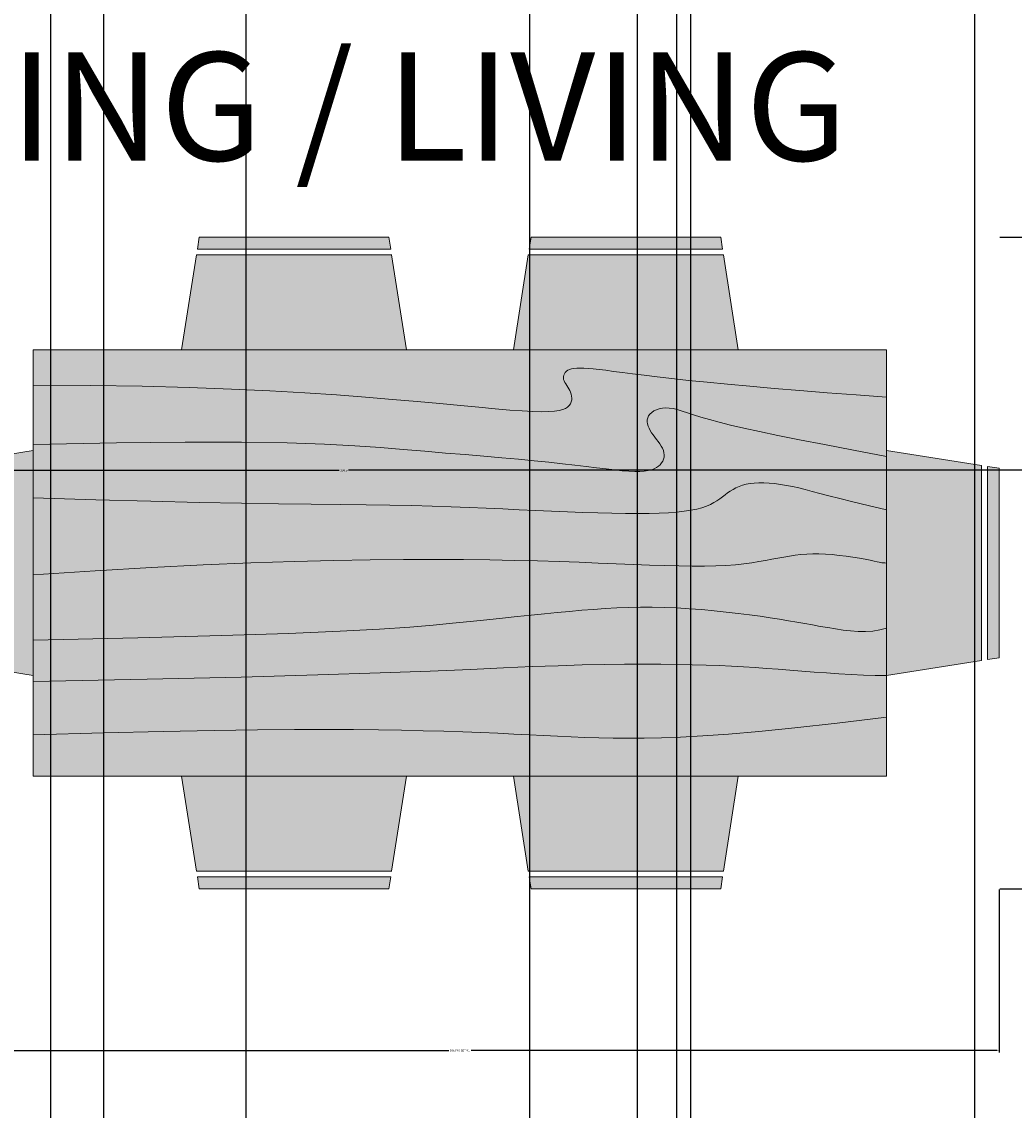
# Model space of a CAD drawing. Units: inches. Extents: x 1434 to 1845, y 1483 to 2014.
# Tile 5 of 11: x 1615 to 1698, y 1737 to 1829. Entities that reach past the tile are written whole.
import ezdxf

# ---------------------------------------------------------------- set-up
doc = ezdxf.new("R2010")
doc.units = ezdxf.units.IN
for name, color, linetype, lineweight in [('A-ANNO-DIMS', 2, 'Continuous', 18), ('A-AREA-IDEN', 7, 'Continuous', 25), ('A-FURN', 9, 'Continuous', 18), ('A-FURN-PATT', 9, 'Continuous', 13)]:
    doc.layers.add(name, color=color, linetype=linetype, lineweight=lineweight)
doc.styles.get("Standard").update_dxf_attribs({"font": 'arial.ttf'})
doc.dimstyles.get("Standard").update_dxf_attribs({"dimtxt": 0.18, "dimasz": 0.18, "dimexe": 0.18, "dimexo": 0.0625, "dimgap": 0.09, "dimtad": 0, "dimtih": 1, "dimtoh": 1, "dimdec": 4, "dimzin": 0, "dimdsep": 46, "dimtxsty": 'Standard', "dimcen": 0.09, "dimadec": 0, "dimazin": 0, "dimtfac": 1, "dimtdec": 4, "dimtofl": 0, "dimtmove": 0, "dimatfit": 3, "dimfxl": 1, "dimtolj": 1, "dimtzin": 0, "dimarcsym": 0})

# ---------------------------------------------------------------- blocks, each defined once
blk = doc.blocks.new('Dining Set - 36 x 72 in.')
for p, q in [((-22, 27.5), (-22.1562, 26.50042)), ((-22, 27.5), (-6, 27.5)), ((-5.8437, 26.49966), (-6, 27.5)), ((6, 27.5), (5.8438, 26.50042)), ((6, 27.5), (22, 27.5)), ((22.1563, 26.49966), (22, 27.5)), ((-22.2343, 26.00059), (-23.4847, 17.99762)), ((-22.2304, 26), (-5.7608, 26)), ((-5.8416, 26.5), (-22.1534, 26.5)), ((-4.5152, 17.99762), (-5.7655, 25.99926)), ((5.7657, 26.00059), (4.5153, 17.99762)), ((5.7696, 26), (22.2392, 26)), ((22.1584, 26.5), (5.8466, 26.5)), ((23.4848, 17.99762), (22.2345, 25.99926)), ((36, 18), (-36, 18)), ((-36, 18), (-36, -18)), ((36, -18), (36, 18)), ((-44.0006, 8.23428), (-35.9976, 9.48474)), ((44.0006, 8.23428), (35.9976, 9.48474)), ((-45.5, 8), (-44.5004, 8.15617)), ((-45.5, 8), (-45.5, -8)), ((-44.5, -8.15843), (-44.5, 8.15338)), ((-44, 8.23041), (-44, -8.23915)), ((44, 8.23041), (44, -8.23915)), ((44.5, -8.15843), (44.5, 8.15338)), ((45.5, 8), (44.5005, 8.15617)), ((45.5, 8), (45.5, -8)), ((-44.4997, -8.15631), (-45.5, -8)), ((-35.9976, -9.48476), (-43.9993, -8.2345)), ((35.9976, -9.48476), (43.9993, -8.2345)), ((44.4997, -8.15631), (45.5, -8)), ((-36, -18), (36, -18)), ((-22.2343, -26.0006), (-23.4847, -17.99762)), ((-4.5152, -17.99762), (-5.7655, -25.99928)), ((5.7657, -26.0006), (4.5153, -17.99762)), ((23.4848, -17.99762), (22.2345, -25.99928)), ((-22.2304, -26), (-5.7608, -26)), ((-22, -27.5), (-22.1562, -26.50044)), ((-5.8416, -26.5), (-22.1534, -26.5)), ((-5.8437, -26.49967), (-6, -27.5)), ((5.7696, -26), (22.2392, -26)), ((6, -27.5), (5.8438, -26.50044)), ((22.1584, -26.5), (5.8466, -26.5)), ((22.1563, -26.49967), (22, -27.5)), ((-22, -27.5), (-6, -27.5)), ((6, -27.5), (22, -27.5))]:
    blk.add_line(p, q)
for points in [[(-36, 15), (-31.1772, 14.97754), (-26.8079, 14.91406), (-22.8538, 14.81543), (-19.276, 14.6875), (-16.0362, 14.53613), (-13.0957, 14.36718), (-10.4159, 14.18652), (-7.9583, 14), (-5.6904, 13.81315), (-3.6035, 13.63021), (-1.6954, 13.45508), (0.0365, 13.29166), (1.5945, 13.14388), (2.9811, 13.01562), (4.1988, 12.9108), (5.25, 12.83333), (6.1393, 12.78613), (6.8802, 12.76823), (7.4883, 12.77767), (7.9792, 12.8125), (8.3685, 12.87077), (8.6719, 12.95052), (8.9049, 13.0498), (9.0833, 13.16666), (9.2205, 13.29899), (9.3216, 13.44401), (9.3895, 13.59879), (9.4271, 13.76041), (9.4373, 13.92594), (9.4232, 14.09245), (9.3875, 14.257), (9.3333, 14.41666), (9.2638, 14.56917), (9.1836, 14.71484), (9.0975, 14.85465), (9.0104, 14.98958), (8.9272, 15.1206), (8.8529, 15.2487), (8.7922, 15.37483), (8.75, 15.5), (8.7305, 15.62467), (8.7344, 15.74739), (8.7617, 15.86621), (8.8125, 15.97916), (8.8867, 16.08431), (8.9844, 16.17968), (9.1055, 16.26334), (9.25, 16.33333), (9.4189, 16.38802), (9.6172, 16.42708), (9.8506, 16.45052), (10.125, 16.45833), (10.4463, 16.45052), (10.8203, 16.42708), (11.2529, 16.38802), (11.75, 16.33333), (12.3184, 16.26318), (12.9694, 16.17838), (13.7151, 16.07991), (14.5677, 15.96875), (15.5395, 15.84586), (16.6426, 15.71224), (17.8893, 15.56884), (19.2917, 15.41666), (20.859, 15.25667), (22.5879, 15.08984), (24.4721, 14.91715), (26.5052, 14.73958), (28.6809, 14.5581), (30.9929, 14.3737), (33.4347, 14.18733), (36, 14)], [(-36, 10), (-28.9766, 10.14274), (-23.1725, 10.20442), (-18.4241, 10.19775), (-14.5677, 10.13541), (-11.4399, 10.03011), (-8.877, 9.89453), (-6.7154, 9.74137), (-4.7917, 9.58333), (-2.9698, 9.43082), (-1.2246, 9.28515), (0.4415, 9.14534), (2.026, 9.01041), (3.5266, 8.87939), (4.9408, 8.7513), (6.266, 8.62516), (7.5, 8.5), (8.6411, 8.37549), (9.6914, 8.2539), (10.6538, 8.13818), (11.5312, 8.03125), (12.3267, 7.93603), (13.043, 7.85547), (13.6831, 7.79248), (14.25, 7.75), (14.7471, 7.7303), (15.1797, 7.73307), (15.5537, 7.75732), (15.875, 7.80208), (16.1494, 7.86637), (16.3828, 7.94922), (16.5811, 8.04964), (16.75, 8.16666), (16.8944, 8.29915), (17.0143, 8.44531), (17.1089, 8.60319), (17.1771, 8.77083), (17.218, 8.94629), (17.2305, 9.1276), (17.2137, 9.31282), (17.1667, 9.5), (17.0895, 9.6875), (16.987, 9.875), (16.8649, 10.0625), (16.7292, 10.25), (16.5856, 10.4375), (16.4401, 10.625), (16.2985, 10.8125), (16.1667, 11), (16.05, 11.18733), (15.9518, 11.3737), (15.8752, 11.5581), (15.8229, 11.73958), (15.798, 11.91715), (15.8034, 12.08984), (15.842, 12.25667), (15.9167, 12.41666), (16.0295, 12.56836), (16.1784, 12.70833), (16.3605, 12.83268), (16.5729, 12.9375), (16.8127, 13.01888), (17.0768, 13.07291), (17.3625, 13.0957), (17.6667, 13.08333), (17.9894, 13.03312), (18.3418, 12.94726), (18.7382, 12.82918), (19.1927, 12.68229), (19.7195, 12.51001), (20.3327, 12.31575), (21.0465, 12.10294), (21.875, 11.875), (22.8357, 11.63354), (23.959, 11.37304), (25.2786, 11.08618), (26.8282, 10.76562), (28.6414, 10.40405), (30.752, 9.99414), (33.1936, 9.52856), (36, 9)], [(-36, 5.5), (-30.7157, 5.3348), (-26.069, 5.20963), (-21.9946, 5.11767), (-18.4271, 5.05208), (-15.3009, 5.00602), (-12.5508, 4.97265), (-10.1112, 4.94515), (-7.9167, 4.91666), (-5.909, 4.88167), (-4.0586, 4.83984), (-2.3429, 4.79215), (-0.7396, 4.73958), (0.7739, 4.6831), (2.22, 4.6237), (3.6213, 4.56233), (5, 4.5), (6.373, 4.43782), (7.7344, 4.3776), (9.0723, 4.32129), (10.375, 4.27083), (11.6309, 4.22819), (12.8281, 4.19531), (13.9551, 4.17415), (15, 4.16666), (15.954, 4.17448), (16.819, 4.19791), (17.6001, 4.23698), (18.3021, 4.29166), (18.9299, 4.36198), (19.4883, 4.44791), (19.9823, 4.54948), (20.4167, 4.66666), (20.7969, 4.79899), (21.1302, 4.94401), (21.4245, 5.09879), (21.6875, 5.26041), (21.9271, 5.42594), (22.1511, 5.59245), (22.3672, 5.757), (22.5834, 5.91666), (22.8065, 6.06868), (23.0404, 6.21093), (23.2879, 6.34147), (23.5521, 6.45833), (23.8358, 6.55957), (24.142, 6.64323), (24.4735, 6.70735), (24.8334, 6.75), (25.2235, 6.76969), (25.642, 6.76692), (26.0858, 6.74267), (26.5521, 6.69791), (27.0379, 6.63362), (27.5404, 6.55078), (28.0565, 6.45036), (28.5834, 6.33333), (29.1242, 6.19987), (29.7071, 6.04687), (30.3661, 5.87044), (31.1354, 5.66666), (32.0493, 5.43164), (33.142, 5.16146), (34.4475, 4.85221), (36, 4.5)], [(-36, -1), (-30.7915, -0.6591), (-26.0195, -0.38216), (-21.6519, -0.16284), (-17.6563, 0.00521), (-14.0005, 0.12833), (-10.6523, 0.21289), (-7.5796, 0.26522), (-4.75, 0.29166), (-2.134, 0.29793), (0.2878, 0.28711), (2.5317, 0.26163), (4.6146, 0.22396), (6.5529, 0.17651), (8.3633, 0.12174), (10.0623, 0.06209), (11.6667, 0), (13.1899, -0.06201), (14.6341, -0.1211), (15.9982, -0.17432), (17.2813, -0.21875), (18.4823, -0.25147), (19.6003, -0.26953), (20.6343, -0.27002), (21.5834, -0.25), (22.4481, -0.20768), (23.2357, -0.14584), (23.9549, -0.06836), (24.6146, 0.02083), (25.2235, 0.11784), (25.7904, 0.21875), (26.3241, 0.31966), (26.8334, 0.41666), (27.3265, 0.50618), (27.8099, 0.58593), (28.2894, 0.65397), (28.7709, 0.70833), (29.2601, 0.74707), (29.763, 0.76823), (30.2855, 0.76985), (30.8334, 0.75), (31.4088, 0.70784), (31.9994, 0.64713), (32.589, 0.57275), (33.1615, 0.48958), (33.7008, 0.4025), (34.1908, 0.3164), (34.6153, 0.23616), (34.9584, 0.16666), (35.2099, 0.11165), (35.3848, 0.07031), (35.504, 0.04069), (35.5886, 0.02083), (35.6594, 0.00879), (35.7377, 0.0026), (35.8442, 0.00032), (36, 0)], [(-36, -6.5), (-27.1843, -6.31267), (-20.084, -6.1263), (-14.469, -5.9419), (-10.1094, -5.76042), (-6.7752, -5.58285), (-4.2363, -5.41016), (-2.2629, -5.24333), (-0.625, -5.08334), (0.8708, -4.93099), (2.2715, -4.78646), (3.5872, -4.64974), (4.8281, -4.52084), (6.0046, -4.39974), (7.127, -4.28646), (8.2053, -4.18099), (9.25, -4.08334), (10.2705, -3.99382), (11.2734, -3.91407), (12.2647, -3.84603), (13.25, -3.79167), (14.2354, -3.75293), (15.2266, -3.73177), (16.2295, -3.73015), (17.25, -3.75), (18.2912, -3.79248), (19.3451, -3.85547), (20.4009, -3.93604), (21.4479, -4.03125), (22.4754, -4.13819), (23.4727, -4.25391), (24.4289, -4.37549), (25.3334, -4.5), (26.1785, -4.62492), (26.9694, -4.74935), (27.7145, -4.87281), (28.4219, -4.99479), (29.1, -5.11483), (29.7572, -5.23242), (30.4016, -5.34709), (31.0417, -5.45834), (31.6837, -5.56437), (32.3262, -5.65821), (32.9658, -5.73153), (33.599, -5.77604), (34.2224, -5.78345), (34.8327, -5.74545), (35.4264, -5.65373), (36, -5.5)], [(-36, -10), (-26.4022, -9.81299), (-18.4675, -9.62891), (-11.9839, -9.45069), (-6.7396, -9.28125), (-2.5226, -9.12354), (0.8789, -8.98047), (3.6769, -8.85498), (6.0833, -8.75), (8.2767, -8.66765), (10.3021, -8.60677), (12.1712, -8.56543), (13.8958, -8.54167), (15.4876, -8.53353), (16.9583, -8.53907), (18.3197, -8.55632), (19.5834, -8.58334), (20.7616, -8.61841), (21.8685, -8.66081), (22.9188, -8.71004), (23.9271, -8.76563), (24.9081, -8.82707), (25.8763, -8.89388), (26.8465, -8.96558), (27.8334, -9.04167), (28.8474, -9.12118), (29.8828, -9.20117), (30.93, -9.27824), (31.9792, -9.34896), (33.0205, -9.40991), (34.0443, -9.45768), (35.0407, -9.48885), (36, -9.5)], [(-36, -14.5), (-30.0881, -14.33513), (-25.0332, -14.21224), (-20.7312, -14.12647), (-17.0781, -14.07292), (-13.97, -14.04671), (-11.3027, -14.04297), (-8.9724, -14.05681), (-6.875, -14.08334), (-4.9224, -14.11833), (-3.0905, -14.16016), (-1.3709, -14.20785), (0.2448, -14.26042), (1.7647, -14.3169), (3.1973, -14.3763), (4.5507, -14.43767), (5.8333, -14.5), (7.0554, -14.5621), (8.235, -14.62175), (9.3922, -14.67652), (10.5469, -14.72396), (11.7192, -14.76164), (12.929, -14.78711), (14.1965, -14.79794), (15.5417, -14.79167), (16.9933, -14.76424), (18.6152, -14.70508), (20.4804, -14.60197), (22.6615, -14.44271), (25.2312, -14.21509), (28.2624, -13.9069), (31.8277, -13.50594), (36, -13)]]:
    blk.add_lwpolyline(points)
blk = doc.blocks.new('*D42')
at = {"layer": 'A-ANNO-DIMS', "color": 0, "lineweight": -2, "transparency": 16777216}
for p, q in [((1606.017, 1755.442), (1606.017, 1741.675)), ((1697.017, 1755.442), (1697.017, 1741.675)), ((1606.197, 1741.855), (1650.566, 1741.855)), ((1696.837, 1741.855), (1652.469, 1741.855))]:
    blk.add_line(p, q, dxfattribs=at)
at = {"layer": 'A-ANNO-DIMS', "color": 0, "transparency": 16777216}
for points in [[(1606.197, 1741.885), (1606.197, 1741.825), (1606.017, 1741.855)], [(1696.837, 1741.885), (1696.837, 1741.825), (1697.017, 1741.855)]]:
    blk.add_solid(points, dxfattribs=at)
at = {"layer": 'Defpoints', "color": 0, "transparency": 16777216}
for p in [(1606.017, 1755.505), (1697.017, 1755.505), (1697.017, 1741.855)]:
    blk.add_point(p, dxfattribs=at)
at = {"layer": 'A-ANNO-DIMS', "color": 0, "transparency": 16777216, "insert": (1651.517, 1741.855), "char_height": 0.18, "attachment_point": 5}
blk.add_mtext('\\A1;DINING SET 91', dxfattribs=at)
blk = doc.blocks.new('*D43')
at = {"layer": 'A-ANNO-DIMS', "color": 0, "lineweight": -2, "transparency": 16777216}
for p, q in [((1697.08, 1810.505), (1710.847, 1810.505)), ((1710.667, 1810.325), (1710.667, 1783.186)), ((1710.667, 1755.685), (1710.667, 1782.823)), ((1697.08, 1755.505), (1710.847, 1755.505))]:
    blk.add_line(p, q, dxfattribs=at)
at = {"layer": 'A-ANNO-DIMS', "color": 0, "transparency": 16777216}
for points in [[(1710.637, 1810.325), (1710.697, 1810.325), (1710.667, 1810.505)], [(1710.637, 1755.685), (1710.697, 1755.685), (1710.667, 1755.505)]]:
    blk.add_solid(points, dxfattribs=at)
at = {"layer": 'Defpoints', "color": 0, "transparency": 16777216}
for p in [(1697.017, 1810.505), (1710.667, 1810.505), (1697.017, 1755.505)]:
    blk.add_point(p, dxfattribs=at)
at = {"layer": 'A-ANNO-DIMS', "color": 0, "transparency": 16777216, "insert": (1710.667, 1783.005), "char_height": 0.18, "attachment_point": 5}
blk.add_mtext('\\A1;55', dxfattribs=at)
blk = doc.blocks.new('*D57')
at = {"layer": 'A-ANNO-DIMS', "color": 0, "lineweight": -2, "transparency": 16777216}
for p, q in [((1616.974, 1974.793), (1616.974, 1483.15)), ((1666.474, 1974.793), (1666.474, 1483.15)), ((1617.154, 1483.33), (1641.396, 1483.33)), ((1666.294, 1483.33), (1642.052, 1483.33))]:
    blk.add_line(p, q, dxfattribs=at)
at = {"layer": 'A-ANNO-DIMS', "color": 0, "transparency": 16777216}
for points in [[(1617.154, 1483.36), (1617.154, 1483.3), (1616.974, 1483.33)], [(1666.294, 1483.36), (1666.294, 1483.3), (1666.474, 1483.33)]]:
    blk.add_solid(points, dxfattribs=at)
at = {"layer": 'Defpoints', "color": 0, "transparency": 16777216}
for p in [(1616.974, 1974.855), (1666.474, 1974.855), (1666.474, 1483.33)]:
    blk.add_point(p, dxfattribs=at)
at = {"layer": 'A-ANNO-DIMS', "color": 0, "transparency": 16777216, "insert": (1641.724, 1483.33), "char_height": 0.18, "attachment_point": 5}
blk.add_mtext('\\A1;49.5', dxfattribs=at)
blk = doc.blocks.new('*D58')
at = {"layer": 'A-ANNO-DIMS', "color": 0, "lineweight": -2, "transparency": 16777216}
for p, q in [((1670.974, 1974.793), (1670.974, 1483.15)), ((1810.474, 1974.793), (1810.474, 1483.15)), ((1671.154, 1483.33), (1740.338, 1483.33)), ((1810.294, 1483.33), (1741.11, 1483.33))]:
    blk.add_line(p, q, dxfattribs=at)
at = {"layer": 'A-ANNO-DIMS', "color": 0, "transparency": 16777216}
for points in [[(1671.154, 1483.36), (1671.154, 1483.3), (1670.974, 1483.33)], [(1810.294, 1483.36), (1810.294, 1483.3), (1810.474, 1483.33)]]:
    blk.add_solid(points, dxfattribs=at)
at = {"layer": 'Defpoints', "color": 0, "transparency": 16777216}
for p in [(1670.974, 1974.855), (1810.474, 1974.855), (1810.474, 1483.33)]:
    blk.add_point(p, dxfattribs=at)
at = {"layer": 'A-ANNO-DIMS', "color": 0, "transparency": 16777216, "insert": (1740.724, 1483.33), "char_height": 0.18, "attachment_point": 5}
blk.add_mtext('\\A1;139.5', dxfattribs=at)
blk = doc.blocks.new('*D62')
at = {"layer": 'A-ANNO-DIMS', "color": 0, "lineweight": -2, "transparency": 16777216}
for p, q in [((1573.474, 1815.793), (1573.474, 1790.65)), ((1709.974, 1815.793), (1709.974, 1790.65)), ((1573.654, 1790.83), (1641.338, 1790.83)), ((1709.794, 1790.83), (1642.11, 1790.83))]:
    blk.add_line(p, q, dxfattribs=at)
at = {"layer": 'A-ANNO-DIMS', "color": 0, "transparency": 16777216}
for points in [[(1573.654, 1790.86), (1573.654, 1790.8), (1573.474, 1790.83)], [(1709.794, 1790.86), (1709.794, 1790.8), (1709.974, 1790.83)]]:
    blk.add_solid(points, dxfattribs=at)
at = {"layer": 'Defpoints', "color": 0, "transparency": 16777216}
for p in [(1573.474, 1815.855), (1709.974, 1815.855), (1573.474, 1790.83)]:
    blk.add_point(p, dxfattribs=at)
at = {"layer": 'A-ANNO-DIMS', "color": 0, "transparency": 16777216, "insert": (1641.724, 1790.83), "char_height": 0.18, "attachment_point": 5}
blk.add_mtext('\\A1;136.5', dxfattribs=at)
blk = doc.blocks.new('*D67')
at = {"layer": 'A-ANNO-DIMS', "color": 0, "lineweight": -2, "transparency": 16777216}
for p, q in [((1694.974, 1517.418), (1694.974, 2013.56)), ((1695.154, 2013.38), (1752.338, 2013.38)), ((1810.294, 2013.38), (1753.11, 2013.38)), ((1810.474, 1517.418), (1810.474, 2013.56))]:
    blk.add_line(p, q, dxfattribs=at)
at = {"layer": 'A-ANNO-DIMS', "color": 0, "transparency": 16777216}
for points in [[(1695.154, 2013.41), (1695.154, 2013.35), (1694.974, 2013.38)], [(1810.294, 2013.41), (1810.294, 2013.35), (1810.474, 2013.38)]]:
    blk.add_solid(points, dxfattribs=at)
at = {"layer": 'Defpoints', "color": 0, "transparency": 16777216}
for p in [(1810.474, 2013.38), (1694.974, 1517.355), (1810.474, 1517.355)]:
    blk.add_point(p, dxfattribs=at)
at = {"layer": 'A-ANNO-DIMS', "color": 0, "transparency": 16777216, "insert": (1752.724, 2013.38), "char_height": 0.18, "attachment_point": 5}
blk.add_mtext('\\A1;115.5', dxfattribs=at)
blk = doc.blocks.new('*D71')
at = {"layer": 'A-ANNO-DIMS', "color": 0, "lineweight": -2, "transparency": 16777216}
for p, q in [((1633.474, 1508.418), (1633.474, 2013.56)), ((1633.654, 2013.38), (1651.253, 2013.38)), ((1669.641, 2013.38), (1652.042, 2013.38)), ((1669.821, 1508.418), (1669.821, 2013.56))]:
    blk.add_line(p, q, dxfattribs=at)
at = {"layer": 'A-ANNO-DIMS', "color": 0, "transparency": 16777216}
for points in [[(1633.654, 2013.41), (1633.654, 2013.35), (1633.474, 2013.38)], [(1669.641, 2013.41), (1669.641, 2013.35), (1669.821, 2013.38)]]:
    blk.add_solid(points, dxfattribs=at)
at = {"layer": 'Defpoints', "color": 0, "transparency": 16777216}
for p in [(1669.821, 2013.38), (1633.474, 1508.355), (1669.821, 1508.355)]:
    blk.add_point(p, dxfattribs=at)
at = {"layer": 'A-ANNO-DIMS', "color": 0, "transparency": 16777216, "insert": (1651.648, 2013.38), "char_height": 0.18, "attachment_point": 5}
blk.add_mtext('\\A1;36.35', dxfattribs=at)
blk = doc.blocks.new('*D72')
at = {"layer": 'A-ANNO-DIMS', "color": 0, "lineweight": -2, "transparency": 16777216}
for p, q in [((1621.474, 1517.418), (1621.474, 2013.56)), ((1621.654, 2013.38), (1627.265, 2013.38)), ((1633.294, 2013.38), (1627.684, 2013.38)), ((1633.474, 1517.418), (1633.474, 2013.56))]:
    blk.add_line(p, q, dxfattribs=at)
at = {"layer": 'A-ANNO-DIMS', "color": 0, "transparency": 16777216}
for points in [[(1621.654, 2013.41), (1621.654, 2013.35), (1621.474, 2013.38)], [(1633.294, 2013.41), (1633.294, 2013.35), (1633.474, 2013.38)]]:
    blk.add_solid(points, dxfattribs=at)
at = {"layer": 'Defpoints', "color": 0, "transparency": 16777216}
for p in [(1633.474, 2013.38), (1621.474, 1517.355), (1633.474, 1517.355)]:
    blk.add_point(p, dxfattribs=at)
at = {"layer": 'A-ANNO-DIMS', "color": 0, "transparency": 16777216, "insert": (1627.474, 2013.38), "char_height": 0.18, "attachment_point": 5}
blk.add_mtext('\\A1;12', dxfattribs=at)
blk = doc.blocks.new('*D86')
at = {"layer": 'A-ANNO-DIMS', "color": 0, "lineweight": -2, "transparency": 16777216}
for p, q in [((1657.378, 1854.658), (1657.378, 1483.15)), ((1666.474, 1854.793), (1666.474, 1483.15)), ((1657.558, 1483.33), (1661.533, 1483.33)), ((1666.294, 1483.33), (1662.32, 1483.33))]:
    blk.add_line(p, q, dxfattribs=at)
at = {"layer": 'A-ANNO-DIMS', "color": 0, "transparency": 16777216}
for points in [[(1657.558, 1483.36), (1657.558, 1483.3), (1657.378, 1483.33)], [(1666.294, 1483.36), (1666.294, 1483.3), (1666.474, 1483.33)]]:
    blk.add_solid(points, dxfattribs=at)
at = {"layer": 'Defpoints', "color": 0, "transparency": 16777216}
for p in [(1657.378, 1854.72), (1666.474, 1854.855), (1657.378, 1483.33)]:
    blk.add_point(p, dxfattribs=at)
at = {"layer": 'A-ANNO-DIMS', "color": 0, "transparency": 16777216, "insert": (1661.926, 1483.33), "char_height": 0.18, "attachment_point": 5}
blk.add_mtext('\\A1;9.096', dxfattribs=at)

msp = doc.modelspace()

# ---------------------------------------------------------------- hatches: boundary and pattern name
at = {"layer": 'A-FURN-PATT'}
h = msp.add_hatch(color=256, dxfattribs=at)
h.dxf.hatch_style = 1
h.paths.add_polyline_path([(1673.6736, 1756.5049), (1657.3611, 1756.5049), (1657.5173, 1755.5049), (1673.5173, 1755.5049)])
h.paths.add_polyline_path([(1645.6736, 1756.5049), (1629.3611, 1756.5049), (1629.5173, 1755.5049), (1645.5173, 1755.5049)])
h.paths.add_polyline_path([(1697.0173, 1791.0049), (1696.0173, 1791.1611), (1696.0173, 1774.8486), (1697.0173, 1775.0049)])
h.paths.add_polyline_path([(1645.5173, 1810.5049), (1629.5173, 1810.5049), (1629.3611, 1809.5049), (1645.6736, 1809.5049)])
h.paths.add_polyline_path([(1673.5173, 1810.5049), (1657.5173, 1810.5049), (1657.3611, 1809.5049), (1673.6736, 1809.5049)])
h.paths.add_polyline_path([(1607.0173, 1791.1611), (1606.0173, 1791.0049), (1606.0173, 1775.0049), (1607.0173, 1774.8486)])
h = msp.add_hatch(color=256, dxfattribs=at)
h.dxf.hatch_style = 1
h.paths.add_polyline_path([(1673.7517, 1809.0049), (1657.2829, 1809.0049), (1656.033, 1801.0049), (1675.0018, 1801.0049)])
h.paths.add_polyline_path([(1645.7517, 1809.0049), (1629.2829, 1809.0049), (1628.033, 1801.0049), (1647.0018, 1801.0049)])
h.paths.add_polyline_path([(1647.0018, 1765.0049), (1628.033, 1765.0049), (1629.2829, 1757.0049), (1645.7517, 1757.0049)])
h.paths.add_polyline_path([(1615.5173, 1792.4892), (1607.5173, 1791.2392), (1607.5173, 1774.7705), (1615.5173, 1773.5205)])
h.paths.add_polyline_path([(1675.0018, 1765.0049), (1656.033, 1765.0049), (1657.2829, 1757.0049), (1673.7517, 1757.0049)])
h.paths.add_polyline_path([(1695.5173, 1791.2392), (1687.5173, 1792.4892), (1687.5173, 1773.5205), (1695.5173, 1774.7705)])
h.paths.add_polyline_path([(1491.9292, 1578.7679), (1493.2417, 1578.7679), (1493.1636, 1579.2679), (1476.6949, 1579.2679), (1476.6168, 1578.7679), (1477.9292, 1578.7679), (1475.9292, 1567.7679, -0.4833507), (1474.5739, 1565.6934), (1474.4292, 1564.7679, 0.4142136), (1475.4292, 1563.7679), (1484.9292, 1563.7679), (1494.4292, 1563.7679, 0.4142136), (1495.4292, 1564.7679), (1495.2846, 1565.6934, -0.4833518), (1493.9292, 1567.7679)])
h.paths.add_polyline_path([(1529.1236, 1578.8204), (1530.4361, 1578.8204), (1530.3579, 1579.3204), (1513.8892, 1579.3204), (1513.8111, 1578.8204), (1515.1236, 1578.8204), (1513.1236, 1567.8204, -0.4833507), (1511.7682, 1565.7459), (1511.6236, 1564.8204, 0.4142136), (1512.6236, 1563.8204), (1522.1236, 1563.8204), (1531.6236, 1563.8204, 0.4142136), (1532.6236, 1564.8204), (1532.4789, 1565.7459, -0.4833518), (1531.1236, 1567.8204)])
h.paths.add_polyline_path([(1531.8672, 1535.8802, -0.4833507), (1533.2226, 1537.9547), (1533.3672, 1538.8802, 0.4142136), (1532.3672, 1539.8802), (1522.8672, 1539.8802), (1513.3672, 1539.8802, 0.4142136), (1512.3672, 1538.8802), (1512.5118, 1537.9547, -0.4833518), (1513.8672, 1535.8802), (1515.8672, 1524.8802), (1514.5547, 1524.8802), (1514.6329, 1524.3802), (1531.1016, 1524.3802), (1531.1797, 1524.8802), (1529.8672, 1524.8802)])
h.paths.add_polyline_path([(1494.3799, 1536.0192, -0.4833507), (1495.7353, 1538.0938), (1495.8799, 1539.0192, 0.4142136), (1494.8799, 1540.0192), (1485.3799, 1540.0192), (1475.8799, 1540.0192, 0.4142136), (1474.8799, 1539.0192), (1475.0245, 1538.0938, -0.4833518), (1476.3799, 1536.0192), (1478.3799, 1525.0193), (1477.0674, 1525.0193), (1477.1456, 1524.5193), (1493.6143, 1524.5193), (1493.6924, 1525.0193), (1492.3799, 1525.0193)])
h = msp.add_hatch(color=256, dxfattribs=at)
h.dxf.hatch_style = 1
h.paths.add_polyline_path([(1660.3268, 1798.3284), (1660.2459, 1798.5685), (1660.2537, 1798.8148), (1660.3561, 1799.0423), (1660.5526, 1799.2342), (1660.7673, 1799.3382), (1660.9362, 1799.3929), (1661.1345, 1799.4319), (1661.3679, 1799.4554), (1661.6423, 1799.4632), (1661.9636, 1799.4554), (1662.3376, 1799.4319), (1662.7702, 1799.3929), (1663.2673, 1799.3382), (1663.8357, 1799.268), (1664.4867, 1799.1832), (1665.2324, 1799.0848), (1666.085, 1798.9736), (1667.0568, 1798.8507), (1668.1599, 1798.7171), (1669.4066, 1798.5737), (1670.809, 1798.4215), (1672.3763, 1798.2615), (1674.1052, 1798.0947), (1675.9894, 1797.922), (1678.0225, 1797.7444), (1680.1982, 1797.563), (1682.5102, 1797.3786), (1684.952, 1797.1922), (1687.5173, 1797.0049), (1687.5173, 1801.0049), (1615.5173, 1801.0049), (1615.5173, 1798.0049), (1620.3401, 1797.9824), (1624.7094, 1797.9189), (1628.6635, 1797.8203), (1632.2413, 1797.6924), (1635.4811, 1797.541), (1638.4216, 1797.372), (1641.1014, 1797.1914), (1643.559, 1797.0049), (1645.8269, 1796.818), (1647.9138, 1796.6351), (1649.8219, 1796.4599), (1651.5538, 1796.2965), (1653.1118, 1796.1487), (1654.4984, 1796.0205), (1655.7161, 1795.9157), (1656.7673, 1795.8382), (1657.6566, 1795.791), (1658.3975, 1795.7731), (1659.0056, 1795.7825), (1659.4965, 1795.8174), (1659.8858, 1795.8756), (1660.1892, 1795.9554), (1660.4222, 1796.0547), (1660.6006, 1796.1715), (1660.7378, 1796.3039), (1660.8389, 1796.4489), (1660.9068, 1796.6037), (1660.9444, 1796.7653), (1660.9546, 1796.9308), (1660.9405, 1797.0973), (1660.9048, 1797.2619), (1660.8506, 1797.4215), (1660.7811, 1797.574), (1660.7009, 1797.7197), (1660.6148, 1797.8595), (1660.4567, 1798.1045)])
h.paths.add_polyline_path([(1668.2465, 1793.2549), (1668.1029, 1793.4424), (1667.8533, 1793.764), (1667.684, 1794.0049), (1667.5673, 1794.1922), (1667.4173, 1794.4768), (1667.3128, 1794.8398), (1667.3235, 1795.1849), (1667.434, 1795.4215), (1667.5468, 1795.5732), (1667.6957, 1795.7132), (1667.8778, 1795.8375), (1668.0902, 1795.9424), (1668.33, 1796.0237), (1668.5941, 1796.0778), (1668.8798, 1796.1006), (1669.184, 1796.0882), (1669.5067, 1796.038), (1669.8591, 1795.9521), (1670.2555, 1795.834), (1670.71, 1795.6872), (1671.2368, 1795.5149), (1671.85, 1795.3206), (1672.5638, 1795.1078), (1673.3923, 1794.8799), (1674.353, 1794.6384), (1675.4763, 1794.3779), (1676.7959, 1794.091), (1678.3455, 1793.7705), (1680.1587, 1793.4089), (1682.2693, 1792.999), (1684.7109, 1792.5334), (1687.5173, 1792.0049), (1687.5173, 1797.0049), (1684.952, 1797.1922), (1682.5102, 1797.3786), (1680.1982, 1797.563), (1678.0225, 1797.7444), (1675.9894, 1797.922), (1674.1052, 1798.0947), (1672.3763, 1798.2615), (1670.809, 1798.4215), (1669.4066, 1798.5737), (1668.1599, 1798.7171), (1667.0568, 1798.8507), (1666.085, 1798.9736), (1665.2324, 1799.0848), (1664.4867, 1799.1832), (1663.8357, 1799.268), (1663.2673, 1799.3382), (1662.7702, 1799.3929), (1662.3376, 1799.4319), (1661.9636, 1799.4554), (1661.6423, 1799.4632), (1661.3679, 1799.4554), (1661.1345, 1799.4319), (1660.9362, 1799.3929), (1660.7673, 1799.3382), (1660.6228, 1799.2682), (1660.5017, 1799.1845), (1660.404, 1799.0892), (1660.3298, 1798.984), (1660.279, 1798.8711), (1660.2517, 1798.7523), (1660.2478, 1798.6295), (1660.2673, 1798.5049), (1660.3095, 1798.3797), (1660.3702, 1798.2536), (1660.4445, 1798.1255), (1660.5277, 1797.9944), (1660.6769, 1797.7634), (1660.8274, 1797.4901), (1660.9338, 1797.1764), (1660.9622, 1796.8416), (1660.8868, 1796.5175), (1660.7378, 1796.3039), (1660.6006, 1796.1715), (1660.4222, 1796.0547), (1660.1892, 1795.9554), (1659.8858, 1795.8756), (1659.4965, 1795.8174), (1659.0056, 1795.7825), (1658.3975, 1795.7731), (1657.6566, 1795.791), (1656.7673, 1795.8382), (1655.7161, 1795.9157), (1654.4984, 1796.0205), (1653.1118, 1796.1487), (1651.5538, 1796.2965), (1649.8219, 1796.4599), (1647.9138, 1796.6351), (1645.8269, 1796.818), (1643.559, 1797.0049), (1641.1014, 1797.1914), (1638.4216, 1797.372), (1635.4811, 1797.541), (1632.2413, 1797.6924), (1628.6635, 1797.8203), (1624.7094, 1797.9189), (1620.3401, 1797.9824), (1615.5173, 1798.0049), (1615.5173, 1793.0049), (1622.5407, 1793.1476), (1628.3448, 1793.2093), (1633.0932, 1793.2026), (1636.9496, 1793.1403), (1640.0774, 1793.035), (1642.6403, 1792.8994), (1644.8019, 1792.7462), (1646.7256, 1792.5882), (1648.5475, 1792.4357), (1650.2927, 1792.29), (1651.9588, 1792.1502), (1653.5433, 1792.0153), (1655.0439, 1791.8843), (1656.4581, 1791.7562), (1657.7833, 1791.63), (1659.0173, 1791.5049), (1660.1584, 1791.3804), (1661.2087, 1791.2588), (1662.1711, 1791.143), (1663.0485, 1791.0361), (1663.844, 1790.9409), (1664.5603, 1790.8603), (1665.2004, 1790.7973), (1665.7673, 1790.7549), (1666.2644, 1790.7352), (1666.697, 1790.7379), (1667.071, 1790.7622), (1667.3923, 1790.8069), (1667.6667, 1790.8712), (1667.9001, 1790.9541), (1668.0984, 1791.0545), (1668.2673, 1791.1715), (1668.4117, 1791.304), (1668.5316, 1791.4502), (1668.6262, 1791.6081), (1668.6944, 1791.7757), (1668.7353, 1791.9512), (1668.7478, 1792.1325), (1668.731, 1792.3177), (1668.684, 1792.5049), (1668.6068, 1792.6924), (1668.5043, 1792.8799), (1668.3822, 1793.0674)])
h.paths.add_polyline_path([(1672.6475, 1787.9489), (1672.9418, 1788.1037), (1673.2048, 1788.2653), (1673.4444, 1788.4308), (1673.6684, 1788.5973), (1673.8845, 1788.7619), (1674.1007, 1788.9215), (1674.3238, 1789.0735), (1674.5577, 1789.2158), (1674.8052, 1789.3463), (1675.0694, 1789.4632), (1675.3531, 1789.5644), (1675.6593, 1789.6481), (1675.9908, 1789.7122), (1676.3507, 1789.7549), (1676.7408, 1789.7746), (1677.1593, 1789.7718), (1677.6031, 1789.7475), (1678.0694, 1789.7028), (1678.5552, 1789.6385), (1679.0577, 1789.5556), (1679.5738, 1789.4552), (1680.1007, 1789.3382), (1680.6415, 1789.2047), (1681.2244, 1789.0517), (1681.8834, 1788.8753), (1682.6527, 1788.6715), (1683.5666, 1788.4365), (1684.6593, 1788.1663), (1685.9648, 1787.8571), (1687.5173, 1787.5049), (1687.5173, 1792.0049), (1684.7109, 1792.5334), (1682.2693, 1792.999), (1680.1587, 1793.4089), (1678.3455, 1793.7705), (1676.7959, 1794.091), (1675.4763, 1794.3779), (1674.353, 1794.6384), (1673.3923, 1794.8799), (1672.5638, 1795.1078), (1671.85, 1795.3206), (1671.2368, 1795.5149), (1670.71, 1795.6872), (1670.2555, 1795.834), (1669.8591, 1795.9521), (1669.5067, 1796.038), (1669.184, 1796.0882), (1668.8798, 1796.1006), (1668.5941, 1796.0778), (1668.33, 1796.0237), (1668.0902, 1795.9424), (1667.8778, 1795.8375), (1667.6957, 1795.7132), (1667.5468, 1795.5732), (1667.434, 1795.4215), (1667.3593, 1795.2615), (1667.3207, 1795.0947), (1667.3153, 1794.922), (1667.3402, 1794.7444), (1667.3925, 1794.563), (1667.4691, 1794.3786), (1667.5673, 1794.1922), (1667.684, 1794.0049), (1667.8158, 1793.8174), (1667.9574, 1793.6299), (1668.1029, 1793.4424), (1668.3374, 1793.1363), (1668.5731, 1792.7742), (1668.684, 1792.5049), (1668.731, 1792.3177), (1668.7562, 1792.0405), (1668.6739, 1791.6876), (1668.5316, 1791.4502), (1668.4117, 1791.304), (1668.2673, 1791.1715), (1668.0984, 1791.0545), (1667.9001, 1790.9541), (1667.6667, 1790.8712), (1667.3923, 1790.8069), (1667.071, 1790.7622), (1666.697, 1790.7379), (1666.2644, 1790.7352), (1665.7673, 1790.7549), (1665.2004, 1790.7973), (1664.5603, 1790.8603), (1663.844, 1790.9409), (1663.0485, 1791.0361), (1662.1711, 1791.143), (1661.2087, 1791.2588), (1660.1584, 1791.3804), (1659.0173, 1791.5049), (1657.7833, 1791.63), (1656.4581, 1791.7562), (1655.0439, 1791.8843), (1653.5433, 1792.0153), (1651.9588, 1792.1502), (1650.2927, 1792.29), (1648.5475, 1792.4357), (1646.7256, 1792.5882), (1644.8019, 1792.7462), (1642.6403, 1792.8994), (1640.0774, 1793.035), (1636.9496, 1793.1403), (1633.0932, 1793.2026), (1628.3448, 1793.2093), (1622.5407, 1793.1476), (1615.5173, 1793.0049), (1615.5173, 1788.5049), (1620.8016, 1788.3397), (1625.4483, 1788.2145), (1629.5227, 1788.1225), (1633.0902, 1788.0569), (1636.2164, 1788.0109), (1638.9665, 1787.9775), (1641.4061, 1787.95), (1643.6006, 1787.9215), (1645.6083, 1787.8865), (1647.4587, 1787.8447), (1649.1744, 1787.797), (1650.7777, 1787.7444), (1652.2912, 1787.688), (1653.7373, 1787.6286), (1655.1386, 1787.5672), (1656.5173, 1787.5049), (1657.8903, 1787.4427), (1659.2517, 1787.3825), (1660.5896, 1787.3262), (1661.8923, 1787.2757), (1663.1482, 1787.2331), (1664.3454, 1787.2002), (1665.4724, 1787.179), (1666.5173, 1787.1715), (1667.4713, 1787.1793), (1668.3363, 1787.2028), (1669.1174, 1787.2418), (1669.8194, 1787.2965), (1670.4472, 1787.3668), (1671.0056, 1787.4528), (1671.4996, 1787.5543), (1671.934, 1787.6715), (1672.3142, 1787.8039)])
h.paths.add_polyline_path([(1687.5173, 1787.5049), (1685.9648, 1787.8571), (1684.6593, 1788.1663), (1683.5666, 1788.4365), (1682.6527, 1788.6715), (1681.8834, 1788.8753), (1681.2244, 1789.0517), (1680.6415, 1789.2047), (1680.1007, 1789.3382), (1679.5738, 1789.4552), (1679.0577, 1789.5556), (1678.5552, 1789.6385), (1678.0694, 1789.7028), (1677.6031, 1789.7475), (1677.1593, 1789.7718), (1676.7408, 1789.7746), (1676.3507, 1789.7549), (1675.9908, 1789.7122), (1675.6593, 1789.6481), (1675.3531, 1789.5644), (1675.0694, 1789.4632), (1674.8052, 1789.3463), (1674.5577, 1789.2158), (1674.3238, 1789.0735), (1674.1007, 1788.9215), (1673.8845, 1788.7619), (1673.6684, 1788.5973), (1673.4444, 1788.4308), (1673.2048, 1788.2653), (1672.9418, 1788.1037), (1672.6475, 1787.9489), (1672.3142, 1787.8039), (1671.934, 1787.6715), (1671.4996, 1787.5543), (1671.0056, 1787.4528), (1670.4472, 1787.3668), (1669.8194, 1787.2965), (1669.1174, 1787.2418), (1668.3363, 1787.2028), (1667.4713, 1787.1793), (1666.5173, 1787.1715), (1665.4724, 1787.179), (1664.3454, 1787.2002), (1663.1482, 1787.2331), (1661.8923, 1787.2757), (1660.5896, 1787.3262), (1659.2517, 1787.3825), (1657.8903, 1787.4427), (1656.5173, 1787.5049), (1655.1386, 1787.5672), (1653.7373, 1787.6286), (1652.2912, 1787.688), (1650.7777, 1787.7444), (1649.1744, 1787.797), (1647.4587, 1787.8447), (1645.6083, 1787.8865), (1643.6006, 1787.9215), (1641.4061, 1787.95), (1638.9665, 1787.9775), (1636.2164, 1788.0109), (1633.0902, 1788.0569), (1629.5227, 1788.1225), (1625.4483, 1788.2145), (1620.8016, 1788.3397), (1615.5173, 1788.5049), (1615.5173, 1782.0049), (1620.7258, 1782.3458), (1625.4978, 1782.6227), (1629.8654, 1782.842), (1633.861, 1783.0101), (1637.5168, 1783.1332), (1640.865, 1783.2178), (1643.9377, 1783.2701), (1646.7673, 1783.2965), (1649.3833, 1783.3028), (1651.8051, 1783.292), (1654.049, 1783.2665), (1656.1319, 1783.2288), (1658.0702, 1783.1814), (1659.8806, 1783.1266), (1661.5796, 1783.067), (1663.184, 1783.0049), (1664.7072, 1782.9429), (1666.1514, 1782.8838), (1667.5155, 1782.8305), (1668.7986, 1782.7861), (1669.9996, 1782.7534), (1671.1176, 1782.7353), (1672.1516, 1782.7348), (1673.1007, 1782.7549), (1673.9654, 1782.7972), (1674.753, 1782.859), (1675.4722, 1782.9365), (1676.1319, 1783.0257), (1676.7408, 1783.1227), (1677.3077, 1783.2236), (1677.8414, 1783.3245), (1678.3507, 1783.4215), (1678.8438, 1783.511), (1679.3272, 1783.5908), (1679.8067, 1783.6588), (1680.2882, 1783.7132), (1680.7774, 1783.7519), (1681.2803, 1783.7731), (1681.8028, 1783.7747), (1682.3507, 1783.7549), (1682.9261, 1783.7127), (1683.5167, 1783.652), (1684.1063, 1783.5776), (1684.6788, 1783.4944), (1685.2181, 1783.4074), (1685.7081, 1783.3213), (1686.1326, 1783.241), (1686.4757, 1783.1715), (1686.7272, 1783.1165), (1686.9021, 1783.0752), (1687.0213, 1783.0456), (1687.1059, 1783.0257), (1687.1767, 1783.0137), (1687.255, 1783.0075), (1687.3615, 1783.0052), (1687.5173, 1783.0049)])
h.paths.add_polyline_path([(1687.5173, 1783.0049), (1687.1918, 1783.0055), (1687.0213, 1783.0456), (1686.9021, 1783.0752), (1686.7272, 1783.1165), (1686.4757, 1783.1715), (1686.1326, 1783.241), (1685.7081, 1783.3213), (1685.2181, 1783.4074), (1684.6788, 1783.4944), (1684.1063, 1783.5776), (1683.5167, 1783.652), (1682.9261, 1783.7127), (1682.3507, 1783.7549), (1681.8028, 1783.7747), (1681.2803, 1783.7731), (1680.7774, 1783.7519), (1680.2882, 1783.7132), (1679.8067, 1783.6588), (1679.3272, 1783.5908), (1678.8438, 1783.511), (1678.3507, 1783.4215), (1677.8414, 1783.3245), (1677.3077, 1783.2236), (1676.7408, 1783.1227), (1676.1319, 1783.0257), (1675.4722, 1782.9365), (1674.753, 1782.859), (1673.9654, 1782.7972), (1673.1007, 1782.7549), (1672.1516, 1782.7348), (1671.1176, 1782.7353), (1669.9996, 1782.7534), (1668.7986, 1782.7861), (1667.5155, 1782.8305), (1666.1514, 1782.8838), (1664.7072, 1782.9429), (1663.184, 1783.0049), (1661.5796, 1783.067), (1659.8806, 1783.1266), (1658.0702, 1783.1814), (1656.1319, 1783.2288), (1654.049, 1783.2665), (1651.8051, 1783.292), (1649.3833, 1783.3028), (1646.7673, 1783.2965), (1643.9377, 1783.2701), (1640.865, 1783.2178), (1637.5168, 1783.1332), (1633.861, 1783.0101), (1629.8654, 1782.842), (1625.4978, 1782.6227), (1620.7258, 1782.3458), (1615.5173, 1782.0049), (1615.5173, 1776.5049), (1624.333, 1776.6922), (1631.4333, 1776.8786), (1637.0483, 1777.063), (1641.4079, 1777.2444), (1644.7421, 1777.422), (1647.281, 1777.5947), (1649.2544, 1777.7615), (1650.8923, 1777.9215), (1652.3881, 1778.0739), (1653.7888, 1778.2184), (1655.1045, 1778.3551), (1656.3454, 1778.484), (1657.5219, 1778.6051), (1658.6443, 1778.7184), (1659.7226, 1778.8239), (1660.7673, 1778.9215), (1661.7878, 1779.011), (1662.7907, 1779.0908), (1663.782, 1779.1588), (1664.7673, 1779.2132), (1665.7527, 1779.2519), (1666.7439, 1779.2731), (1667.7468, 1779.2747), (1668.7673, 1779.2549), (1669.8085, 1779.2124), (1670.8624, 1779.1494), (1671.9182, 1779.0688), (1672.9652, 1778.9736), (1673.9927, 1778.8667), (1674.99, 1778.751), (1675.9462, 1778.6294), (1676.8507, 1778.5049), (1677.6958, 1778.3799), (1678.4867, 1778.2555), (1679.2318, 1778.1321), (1679.9392, 1778.0101), (1680.6173, 1777.89), (1681.2745, 1777.7724), (1681.9189, 1777.6578), (1682.559, 1777.5465), (1683.201, 1777.4405), (1683.8435, 1777.3467), (1684.4831, 1777.2733), (1685.1163, 1777.2288), (1685.7397, 1777.2214), (1686.35, 1777.2594), (1686.9437, 1777.3511), (1687.5173, 1777.5049)])
h.paths.add_polyline_path([(1687.5173, 1777.5049), (1686.9437, 1777.3511), (1686.35, 1777.2594), (1685.7397, 1777.2214), (1685.1163, 1777.2288), (1684.4831, 1777.2733), (1683.8435, 1777.3467), (1683.201, 1777.4405), (1682.559, 1777.5465), (1681.9189, 1777.6578), (1681.2745, 1777.7724), (1680.6173, 1777.89), (1679.9392, 1778.0101), (1679.2318, 1778.1321), (1678.4867, 1778.2555), (1677.6958, 1778.3799), (1676.8507, 1778.5049), (1675.9462, 1778.6294), (1674.99, 1778.751), (1673.9927, 1778.8667), (1672.9652, 1778.9736), (1671.9182, 1779.0688), (1670.8624, 1779.1494), (1669.8085, 1779.2124), (1668.7673, 1779.2549), (1667.7468, 1779.2747), (1666.7439, 1779.2731), (1665.7527, 1779.2519), (1664.7673, 1779.2132), (1663.782, 1779.1588), (1662.7907, 1779.0908), (1661.7878, 1779.011), (1660.7673, 1778.9215), (1659.7226, 1778.8239), (1658.6443, 1778.7184), (1657.5219, 1778.6051), (1656.3454, 1778.484), (1655.1045, 1778.3551), (1653.7888, 1778.2184), (1652.3881, 1778.0739), (1650.8923, 1777.9215), (1649.2544, 1777.7615), (1647.281, 1777.5947), (1644.7421, 1777.422), (1641.4079, 1777.2444), (1637.0483, 1777.063), (1631.4333, 1776.8786), (1624.333, 1776.6922), (1615.5173, 1776.5049), (1615.5173, 1773.0049), (1625.1151, 1773.1919), (1633.0498, 1773.376), (1639.5334, 1773.5542), (1644.7777, 1773.7236), (1648.9947, 1773.8813), (1652.3962, 1774.0244), (1655.1942, 1774.1499), (1657.6006, 1774.2549), (1659.794, 1774.3372), (1661.8194, 1774.3981), (1663.6885, 1774.4394), (1665.4131, 1774.4632), (1667.0049, 1774.4713), (1668.4756, 1774.4658), (1669.837, 1774.4485), (1671.1007, 1774.4215), (1672.2789, 1774.3865), (1673.3858, 1774.3441), (1674.4361, 1774.2948), (1675.4444, 1774.2392), (1676.4254, 1774.1778), (1677.3936, 1774.111), (1678.3638, 1774.0393), (1679.3507, 1773.9632), (1680.3647, 1773.8837), (1681.4001, 1773.8037), (1682.4473, 1773.7266), (1683.4965, 1773.6559), (1684.5378, 1773.595), (1685.5616, 1773.5472), (1686.558, 1773.516), (1687.4243, 1773.5059), (1687.5173, 1773.5205)])
h.paths.add_polyline_path([(1687.5173, 1773.5049), (1686.558, 1773.516), (1685.5616, 1773.5472), (1684.5378, 1773.595), (1683.4965, 1773.6559), (1682.4473, 1773.7266), (1681.4001, 1773.8037), (1680.3647, 1773.8837), (1679.3507, 1773.9632), (1678.3638, 1774.0393), (1677.3936, 1774.111), (1676.4254, 1774.1778), (1675.4444, 1774.2392), (1674.4361, 1774.2948), (1673.3858, 1774.3441), (1672.2789, 1774.3865), (1671.1007, 1774.4215), (1669.837, 1774.4485), (1668.4756, 1774.4658), (1667.0049, 1774.4713), (1665.4131, 1774.4632), (1663.6885, 1774.4394), (1661.8194, 1774.3981), (1659.794, 1774.3372), (1657.6006, 1774.2549), (1655.1942, 1774.1499), (1652.3962, 1774.0244), (1648.9947, 1773.8813), (1644.7777, 1773.7236), (1639.5334, 1773.5542), (1633.0498, 1773.376), (1625.1151, 1773.1919), (1615.5173, 1773.0049), (1615.5173, 1768.5049), (1621.4292, 1768.6697), (1626.4841, 1768.7926), (1630.7861, 1768.8784), (1634.4392, 1768.9319), (1637.5473, 1768.9582), (1640.2146, 1768.9619), (1642.5449, 1768.9481), (1644.6423, 1768.9215), (1646.5949, 1768.8865), (1648.4268, 1768.8447), (1650.1464, 1768.797), (1651.7621, 1768.7444), (1653.282, 1768.688), (1654.7146, 1768.6286), (1656.068, 1768.5672), (1657.3506, 1768.5049), (1658.5727, 1768.4428), (1659.7523, 1768.3831), (1660.9095, 1768.3283), (1662.0642, 1768.2809), (1663.2365, 1768.2432), (1664.4463, 1768.2178), (1665.7138, 1768.2069), (1667.059, 1768.2132), (1668.5106, 1768.2406), (1670.1325, 1768.2998), (1671.9977, 1768.4029), (1674.1788, 1768.5622), (1676.7485, 1768.7898), (1679.7797, 1769.098), (1683.345, 1769.4989), (1687.5173, 1770.0049)])
h.paths.add_polyline_path([(1687.5173, 1770.0049), (1683.345, 1769.4989), (1679.7797, 1769.098), (1676.7485, 1768.7898), (1674.1788, 1768.5622), (1671.9977, 1768.4029), (1670.1325, 1768.2998), (1668.5106, 1768.2406), (1667.059, 1768.2132), (1665.7138, 1768.2069), (1664.4463, 1768.2178), (1663.2365, 1768.2432), (1662.0642, 1768.2809), (1660.9095, 1768.3283), (1659.7523, 1768.3831), (1658.5727, 1768.4428), (1657.3506, 1768.5049), (1656.068, 1768.5672), (1654.7146, 1768.6286), (1653.282, 1768.688), (1651.7621, 1768.7444), (1650.1464, 1768.797), (1648.4268, 1768.8447), (1646.5949, 1768.8865), (1644.6423, 1768.9215), (1642.5449, 1768.9481), (1640.2146, 1768.9619), (1637.5473, 1768.9582), (1634.4392, 1768.9319), (1630.7861, 1768.8784), (1626.4841, 1768.7926), (1621.4292, 1768.6697), (1615.5173, 1768.5049), (1615.5173, 1765.0049), (1687.5173, 1765.0049)])

# ---------------------------------------------------------------- block references
at = {"layer": 'A-FURN'}
msp.add_blockref('Dining Set - 36 x 72 in.', (1651.5173, 1783.0049), dxfattribs=at)

# ---------------------------------------------------------------- texts
at = {"layer": 'A-AREA-IDEN'}
msp.add_text('DINING / LIVING ', height=9.146682, dxfattribs=at).set_placement((1592.3026, 1816.9675))

# ---------------------------------------------------------------- dimensions: what is measured, and where the dimension line sits
at = {"layer": 'A-ANNO-DIMS'}
for base, p1, p2, override, picture, middle in [((1633.4742, 2013.3803), (1621.4742, 1517.3553), (1633.4742, 1517.3553), {"dimdec": 0, "dimlfac": 1, "dimrnd": 0, "dimzin": 0, "dimdsep": 46, "dimlunit": 2}, '*D72', (1627.4742, 2013.3803)), ((1669.8212, 2013.3803), (1633.4742, 1508.3553), (1669.8212, 1508.3553), {"dimdec": 2, "dimlfac": 1, "dimrnd": 0, "dimzin": 0, "dimdsep": 46, "dimlunit": 2}, '*D71', (1651.6477, 2013.3803)), ((1810.4742, 2013.3803), (1694.9742, 1517.3553), (1810.4742, 1517.3553), {"dimdec": 1, "dimlfac": 1, "dimrnd": 0, "dimzin": 0, "dimdsep": 46, "dimlunit": 2}, '*D67', (1752.7242, 2013.3803)), ((1666.4742, 1483.3303), (1616.9742, 1974.8553), (1666.4742, 1974.8553), {"dimdec": 1, "dimlfac": 1, "dimrnd": 0, "dimzin": 0, "dimdsep": 46, "dimlunit": 2}, '*D57', (1641.7242, 1483.3303)), ((1810.4742, 1483.3303), (1670.9742, 1974.8553), (1810.4742, 1974.8553), {"dimdec": 1, "dimlfac": 1, "dimrnd": 0, "dimzin": 0, "dimdsep": 46, "dimlunit": 2}, '*D58', (1740.7242, 1483.3303)), ((1657.3781, 1483.3303), (1666.4742, 1854.8553), (1657.3781, 1854.7205), {"dimdec": 3, "dimlfac": 1, "dimrnd": 0, "dimzin": 0, "dimdsep": 46, "dimlunit": 2}, '*D86', (1661.9261, 1483.3303))]:
    dim = msp.add_linear_dim(base=base, p1=p1, p2=p2, dimstyle='Standard', override=override, dxfattribs=at)
    dim.commit()
    dim.dimension.update_dxf_attribs({"geometry": picture, "text_midpoint": middle})
for base, p1, p2, angle, override, picture, middle in [((1573.4742, 1790.8303), (1709.9742, 1815.8553), (1573.4742, 1815.8553), 180, {"dimdec": 1, "dimlfac": 1, "dimrnd": 0, "dimzin": 0, "dimdsep": 46, "dimlunit": 2}, '*D62', (1641.7242, 1790.8303)), ((1710.6673, 1810.5049), (1697.0173, 1755.5049), (1697.0173, 1810.5049), 90, {"dimdec": 0, "dimlfac": 1, "dimrnd": 0, "dimzin": 0, "dimdsep": 46, "dimlunit": 2}, '*D43', (1710.6673, 1783.0049))]:
    dim = msp.add_linear_dim(base=base, p1=p1, p2=p2, angle=angle, dimstyle='Standard', override=override, dxfattribs=at)
    dim.commit()
    dim.dimension.update_dxf_attribs({"geometry": picture, "text_midpoint": middle})
dim = msp.add_linear_dim(base=(1697.0173, 1741.8549), p1=(1606.0173, 1755.5049), p2=(1697.0173, 1755.5049), text='DINING SET <>', dimstyle='Standard', override={"dimdec": 0, "dimlfac": 1, "dimrnd": 0, "dimzin": 0, "dimdsep": 46, "dimlunit": 2}, dxfattribs=at)
dim.commit()
dim.dimension.update_dxf_attribs({"geometry": '*D42', "text_midpoint": (1651.5173, 1741.8549)})

doc.saveas('drawing.dxf')
